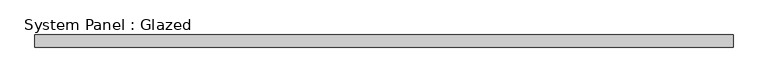
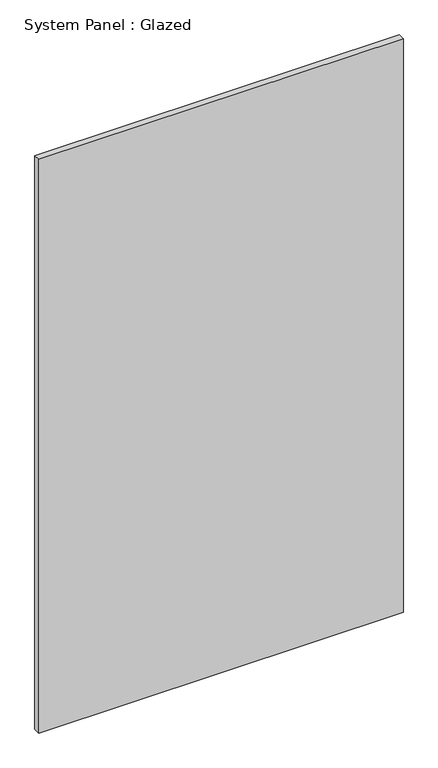
"""IFC4 building model written with IfcOpenShell, lengths in millimetres: plate geometry, System Panel : Glazed."""

from ifc_helpers import new_model, si_unit, origin, origin_with_axes, place, context, project, spatial, polyline, outline, extrude, source, transform, mapped, element, save


def system_panel_glazed_58f29689(model_context):
    return source(origin(), model_context, "Body", "SweptSolid", [
        extrude(outline(polyline([(704.85, 19.05), (-704.85, 19.05), (-704.85, 44.45), (704.85, 44.45), (704.85, 19.05)])), origin_with_axes(), (0.0, 0.0, 1.0), 2343.15),
    ])


if __name__ == "__main__":
    model = new_model("IFC4")
    model_context = context("Model", 3, world=origin())
    ifc_project = project(units=[si_unit("LENGTHUNIT", "METRE", prefix="MILLI")], contexts=[model_context])
    site = spatial("IfcSite", under=ifc_project)
    building = spatial("IfcBuilding", under=site)
    placement = place(None, origin())
    system_panel_glazed_shape = system_panel_glazed_58f29689(model_context)
    element("IfcPlate", 1, ObjectType="System Panel : Glazed", at=placement, inside=building, context=model_context, shape_type="MappedRepresentation", body=[
        mapped(system_panel_glazed_shape, transform((0.0, 0.0, 0.0), x_axis=(1.0, 0.0, 0.0), y_axis=(0.0, 1.0, 0.0), z_axis=(0.0, 0.0, 1.0))),
    ])
    save(model, "model.ifc")

# Revit data of these elements
# Type "System Panel : Glazed"
#   Construction Type Id = "GSP4R"
#   Analytic Construction = "1/8 in Pilkington single glazing"
#   Visual Light Transmittance = 0.9
#   Solar Heat Gain Coefficient = 0.86
#   Heat Transfer Coefficient (U) = 1.18115 BTU/(h·ft²·°F)
# Element 1 (IfcPlate, "System Panel : Glazed")
#   Materials on its faces: "Glass"
# Materials
#   "Glass": class "Glass", colour RGB 0 128 192, transparency 0.75, Description = "Soda Lime Glass", Cost = 0
